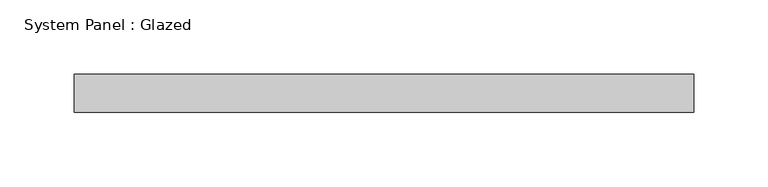
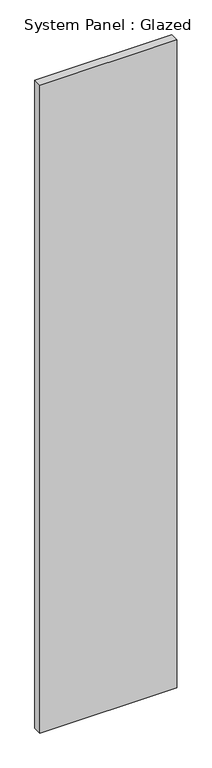
"""IFC4 building model written with IfcOpenShell, lengths in millimetres: plate geometry, System Panel : Glazed."""

from ifc_helpers import new_model, si_unit, origin, origin_with_axes, place, context, project, spatial, polyline, outline, extrude, source, transform, mapped, element, save


def system_panel_glazed_b4366bb5(model_context):
    return source(origin(), model_context, "Body", "SweptSolid", [
        extrude(outline(polyline([(208.3239274, 19.05), (-208.3239274, 19.05), (-208.3239274, 44.45), (208.3239274, 44.45), (208.3239274, 19.05)])), origin_with_axes(), (0.0, 0.0, 1.0), 2082.8),
    ])


if __name__ == "__main__":
    model = new_model("IFC4")
    model_context = context("Model", 3, world=origin())
    ifc_project = project(units=[si_unit("LENGTHUNIT", "METRE", prefix="MILLI")], contexts=[model_context])
    site = spatial("IfcSite", under=ifc_project)
    building = spatial("IfcBuilding", under=site)
    placement = place(None, origin())
    system_panel_glazed_shape = system_panel_glazed_b4366bb5(model_context)
    element("IfcPlate", 1, ObjectType="System Panel : Glazed", at=placement, inside=building, context=model_context, shape_type="MappedRepresentation", body=[
        mapped(system_panel_glazed_shape, transform((0.0, 0.0, 0.0), x_axis=(1.0, 0.0, 0.0), y_axis=(0.0, 1.0, 0.0), z_axis=(0.0, 0.0, 1.0))),
    ])
    save(model, "model.ifc")

# Revit data of these elements
# Type "System Panel : Glazed"
#   Construction Type Id = "GSP4R"
#   Analytic Construction = "1/8 in Pilkington single glazing"
#   Visual Light Transmittance = 0.9
#   Solar Heat Gain Coefficient = 0.86
#   Heat Transfer Coefficient (U) = 1.18115 BTU/(h·ft²·°F)
#   Define Thermal Properties by = 1
# Element 1 (IfcPlate, "System Panel : Glazed")
#   Materials on its faces: "Glass"
# Materials
#   "Glass": class "Glass", colour RGB 0 128 192, transparency 0.75, Description = "Soda Lime Glass", Cost = 0
